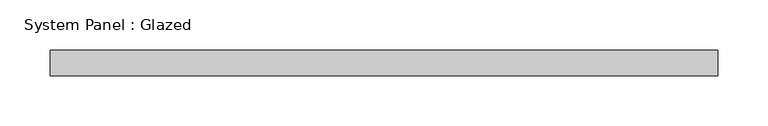
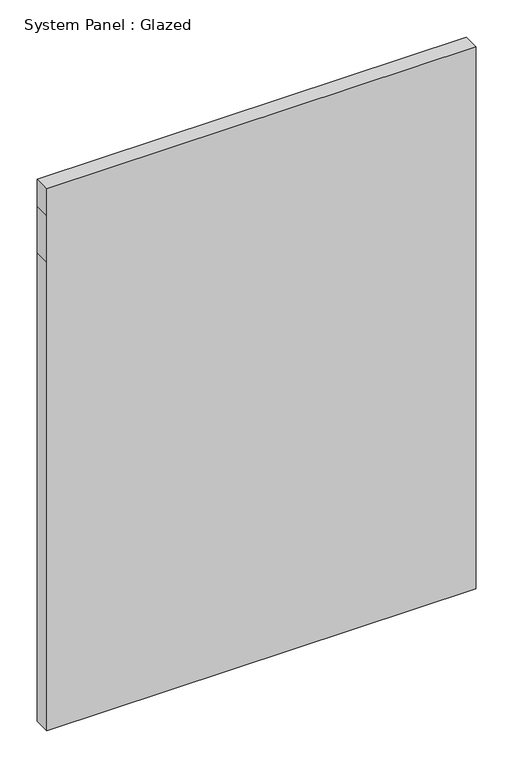
"""IFC4 building model written with IfcOpenShell, lengths in millimetres: plate geometry, System Panel : Glazed."""

from ifc_helpers import new_model, si_unit, frame, origin, place, context, project, spatial, polyline, outline, extrude, source, transform, mapped, element, save


def system_panel_glazed_cfa4a589(model_context):
    return source(origin(), model_context, "Body", "SweptSolid", [
        extrude(outline(polyline([(0.0, -333.375), (0.0, 333.375), (768.9388769, 333.375), (845.1388769, 333.375), (889.5888769, 333.375), (889.5888769, -333.375), (845.1388769, -333.375), (768.9388769, -333.375), (0.0, -333.375)])), frame((0.0, 19.05, 0.0), z_axis=(0.0, 1.0, 0.0), x_axis=(0.0, 0.0, 1.0)), (0.0, 0.0, 1.0), 25.4),
    ])


if __name__ == "__main__":
    model = new_model("IFC4")
    model_context = context("Model", 3, world=origin())
    ifc_project = project(units=[si_unit("LENGTHUNIT", "METRE", prefix="MILLI")], contexts=[model_context])
    site = spatial("IfcSite", under=ifc_project)
    building = spatial("IfcBuilding", under=site)
    placement = place(None, origin())
    system_panel_glazed_shape = system_panel_glazed_cfa4a589(model_context)
    element("IfcPlate", 1, ObjectType="System Panel : Glazed", at=placement, inside=building, context=model_context, shape_type="MappedRepresentation", body=[
        mapped(system_panel_glazed_shape, transform((0.0, 0.0, 0.0), x_axis=(1.0, 0.0, 0.0), y_axis=(0.0, 1.0, 0.0), z_axis=(0.0, 0.0, 1.0))),
    ])
    save(model, "model.ifc")

# Revit data of these elements
# Type "System Panel : Glazed"
#   Construction Type Id = "GSP4R"
#   Analytic Construction = "1/8 in Pilkington single glazing"
#   Visual Light Transmittance = 0.9
#   Solar Heat Gain Coefficient = 0.86
#   Heat Transfer Coefficient (U) = 1.18115 BTU/(h·ft²·°F)
#   Define Thermal Properties by = 1
# Element 1 (IfcPlate, "System Panel : Glazed")
#   Materials on its faces: "Glass"
# Materials
#   "Glass": class "Glass", colour RGB 0 128 192, transparency 0.75, Description = "Soda Lime Glass", Cost = 0
